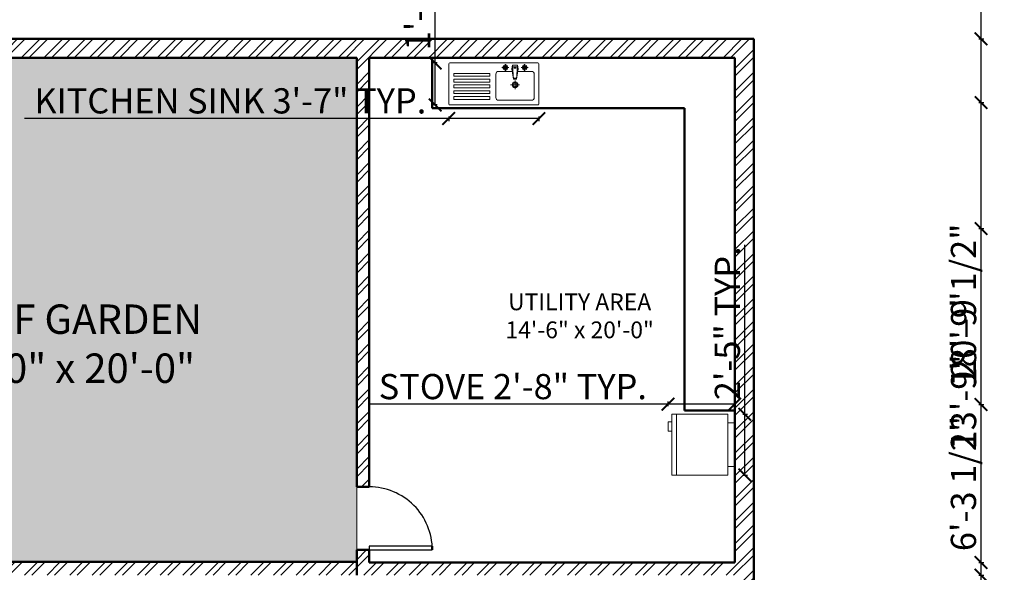
# Model space of a CAD drawing. Units: inches. Extents: x 261 to 2725, y 291 to 1454.
# Tile 34 of 35: x 2144 to 2613, y 801 to 1064. Entities that reach past the tile are written whole.
import ezdxf

# ---------------------------------------------------------------- set-up
doc = ezdxf.new("R2010")
doc.units = ezdxf.units.IN
for name, color, linetype, lineweight in [('A-ANNO-DIMS', 136, 'Continuous', 18), ('A-AREA-IDEN', 18, 'Continuous', 18), ('A-DOOR', 160, 'Continuous', 25), ('A-FLOR-FIXT', 145, 'Continuous', 18), ('A-PLNT', 3, 'Continuous', 18), ('A-PLNT-PATT', 3, 'Continuous', 13), ('A-WALL', 222, 'Continuous', 50), ('A-WALL-PATT', 243, 'Continuous', 13)]:
    doc.layers.add(name, color=color, linetype=linetype, lineweight=lineweight)
doc.styles.get("Standard").update_dxf_attribs({"font": 'arial.ttf'})
doc.dimstyles.new('ISO-25', dxfattribs={"dimtxt": 12, "dimasz": 6, "dimexe": 1.25, "dimexo": 0.625, "dimtad": 1, "dimdec": 0, "dimlunit": 3, "dimtxsty": 'Standard', "dimblk": 'ARCHTICK', "dimcen": 2.5, "dimadec": 0, "dimazin": 0, "dimtfac": 1, "dimtdec": 0, "dimtmove": 0, "dimatfit": 3, "dimfxl": 1, "dimfxlon": 1, "dimarcsym": 0})

# ---------------------------------------------------------------- blocks, each defined once
blk = doc.blocks.new('*U9')
for p, q in [((0, 0), (0, 6)), ((30, 0), (30, 6))]:
    blk.add_line(p, q)
blk.add_lwpolyline([(0, 0), (0, -30), (1.75, -30), (1.75, 0)], close=True)
blk.add_arc((0, 0), 30, 270, 0)
blk = doc.blocks.new('A$C7C492201')
for p, q in [((0, 10), (0, 427)), ((10, 437), (927, 437)), ((148, 425), (148, 352)), ((223, 415), (217, 376)), ((223, 415), (232, 268)), ((223, 415), (248, 415)), ((273, 415), (248, 415)), ((273, 415), (265, 268)), ((273, 415), (280, 376)), ((348, 425), (348, 352)), ((937, 10), (937, 427)), ((48, 319), (48, 79)), ((221, 349), (78, 349)), ((112, 389), (185, 389)), ((217, 376), (232, 268)), ((225, 395), (248, 395)), ((272, 395), (248, 395)), ((280, 376), (265, 268)), ((418, 349), (276, 349)), ((312, 389), (385, 389)), ((448, 319), (448, 79)), ((509, 328), (509, 298)), ((509, 328), (885, 328)), ((885, 328), (885, 298)), ((203, 208), (294, 208)), ((231, 279), (248, 279)), ((232, 268), (248, 268)), ((266, 279), (248, 279)), ((265, 268), (248, 268)), ((248, 253), (248, 163)), ((509, 298), (885, 298)), ((509, 268), (509, 238)), ((509, 268), (885, 268)), ((509, 238), (885, 238)), ((509, 208), (885, 208)), ((509, 208), (509, 178)), ((885, 268), (885, 238)), ((885, 208), (885, 178)), ((509, 178), (885, 178)), ((509, 148), (509, 118)), ((509, 148), (885, 148)), ((509, 118), (885, 118)), ((885, 148), (885, 118)), ((927, 0), (10, 0)), ((418, 49), (78, 49)), ((509, 88), (509, 58)), ((509, 88), (885, 88)), ((509, 58), (885, 58)), ((885, 88), (885, 58))]:
    blk.add_line(p, q)
for centre, radius in [((148, 389), 25), ((348, 389), 25), ((148, 389), 15), ((348, 389), 15), ((248, 208), 30), ((248, 208), 20)]:
    blk.add_circle(centre, radius)
for centre, radius, start, end in [((10, 427), 10, 90, 180), ((927, 427), 10, 0, 90), ((78, 319), 30, 90, 180), ((247, 388), 7.19, 80.5252, 279.4748), ((250, 388), 7.19, 260.5252, 99.4748), ((418, 319), 30, 0, 90), ((10, 10), 10, 180, 270), ((78, 79), 30, 180, 270), ((418, 79), 30, 270, 0), ((927, 10), 10, 270, 0)]:
    blk.add_arc(centre, radius, start, end)
blk = doc.blocks.new('A$C659B0DF6')
for p, q in [((585, 606.1), (0, 606.1)), ((0, 66.1), (0, 606.1)), ((423, 642.1), (423, 606.1)), ((513, 642.1), (423, 642.1)), ((513, 606.1), (513, 642.1)), ((585, 66.1), (585, 606.1)), ((585, 561.1), (0, 561.1)), ((0, 66.1), (585, 66.1)), ((82.3, 0), (82.3, 66.1)), ((502.7, 0), (502.7, 66.1)), ((82.3, 0), (502.7, 0))]:
    blk.add_line(p, q)
blk = doc.blocks.new('_ArchTick')
at = {"color": 0, "linetype": 'ByBlock', "const_width": 0.15}
blk.add_lwpolyline([(-0.5, -0.5), (0.5, 0.5)], dxfattribs=at)
blk = doc.blocks.new('*D51')
at = {"layer": 'A-ANNO-DIMS', "color": 0, "lineweight": -2, "ltscale": 0.07, "transparency": 16777216}
for p, q in [((2348.5, 1017.91), (2348.5, 1015.66)), ((2391.44, 1017.91), (2391.44, 1015.66)), ((2348.5, 1016.91), (2146.62, 1016.91)), ((2391.44, 1016.91), (2348.5, 1016.91))]:
    blk.add_line(p, q, dxfattribs=at)
at = {"layer": 'Defpoints', "color": 0, "ltscale": 0.07, "transparency": 16777216}
for p in [(2348.5, 1023.35), (2391.44, 1023.35), (2348.5, 1016.91)]:
    blk.add_point(p, dxfattribs=at)
at = {"layer": 'A-ANNO-DIMS', "color": 0, "lineweight": -2, "ltscale": 0.07, "transparency": 16777216, "xscale": 6, "yscale": 6, "zscale": 6, "rotation": 180}
blk.add_blockref('_ArchTick', (2348.5, 1016.91), dxfattribs=at)
at = {"layer": 'A-ANNO-DIMS', "color": 0, "lineweight": -2, "ltscale": 0.07, "transparency": 16777216, "xscale": 6, "yscale": 6, "zscale": 6}
blk.add_blockref('_ArchTick', (2391.44, 1016.91), dxfattribs=at)
at = {"layer": 'A-ANNO-DIMS', "color": 0, "ltscale": 0.07, "transparency": 16777216, "insert": (2244.56, 1023.75), "char_height": 12, "attachment_point": 5}
blk.add_mtext('KITCHEN SINK 3\'-7" TYP.', dxfattribs=at)
blk = doc.blocks.new('*D52')
at = {"layer": 'A-ANNO-DIMS', "color": 0, "lineweight": -2, "ltscale": 0.07, "transparency": 16777216}
for p, q in [((2342.06, 1043.35), (2342.06, 1122.62)), ((2343.06, 1043.35), (2340.81, 1043.35)), ((2342.06, 1023.35), (2342.06, 1043.35)), ((2343.06, 1023.35), (2340.81, 1023.35))]:
    blk.add_line(p, q, dxfattribs=at)
at = {"layer": 'Defpoints', "color": 0, "ltscale": 0.07, "transparency": 16777216}
for p in [(2342.06, 1043.35), (2348.5, 1043.35), (2348.5, 1023.35)]:
    blk.add_point(p, dxfattribs=at)
at = {"layer": 'A-ANNO-DIMS', "color": 0, "lineweight": -2, "ltscale": 0.07, "transparency": 16777216, "xscale": 6, "yscale": 6, "zscale": 6}
for p, rotation in [((2342.06, 1043.35), 90), ((2342.06, 1023.35), 270)]:
    blk.add_blockref('_ArchTick', p, dxfattribs=dict(at, rotation=rotation))
at = {"layer": 'A-ANNO-DIMS', "color": 0, "ltscale": 0.07, "transparency": 16777216, "insert": (2335.31, 1085.99), "char_height": 12, "attachment_point": 5, "rotation": 90}
blk.add_mtext('1\'-8" TYP.', dxfattribs=at)
blk = doc.blocks.new('*D53')
at = {"layer": 'A-ANNO-DIMS', "color": 0, "lineweight": -2, "ltscale": 0.07, "transparency": 16777216}
for p, q in [((2452.93, 879.86), (2452.93, 882.11)), ((2484.71, 879.86), (2484.71, 882.11)), ((2452.93, 880.86), (2311.11, 880.86)), ((2484.71, 880.86), (2452.93, 880.86))]:
    blk.add_line(p, q, dxfattribs=at)
at = {"layer": 'Defpoints', "color": 0, "ltscale": 0.07, "transparency": 16777216}
for p in [(2452.93, 880.86), (2452.93, 876.09), (2484.71, 876.09)]:
    blk.add_point(p, dxfattribs=at)
at = {"layer": 'A-ANNO-DIMS', "color": 0, "lineweight": -2, "ltscale": 0.07, "transparency": 16777216, "xscale": 6, "yscale": 6, "zscale": 6, "rotation": 180}
blk.add_blockref('_ArchTick', (2452.93, 880.86), dxfattribs=at)
at = {"layer": 'A-ANNO-DIMS', "color": 0, "lineweight": -2, "ltscale": 0.07, "transparency": 16777216, "xscale": 6, "yscale": 6, "zscale": 6}
blk.add_blockref('_ArchTick', (2484.71, 880.86), dxfattribs=at)
at = {"layer": 'A-ANNO-DIMS', "color": 0, "ltscale": 0.07, "transparency": 16777216, "insert": (2379.02, 887.69), "char_height": 12, "attachment_point": 5}
blk.add_mtext('STOVE 2\'-8" TYP.', dxfattribs=at)
blk = doc.blocks.new('*D54')
at = {"layer": 'A-ANNO-DIMS', "color": 0, "lineweight": -2, "ltscale": 0.07, "transparency": 16777216}
for p, q in [((2489.47, 876.09), (2489.47, 956.69)), ((2488.47, 876.09), (2490.72, 876.09)), ((2489.47, 847.13), (2489.47, 876.09)), ((2488.47, 847.13), (2490.72, 847.13))]:
    blk.add_line(p, q, dxfattribs=at)
at = {"layer": 'Defpoints', "color": 0, "ltscale": 0.07, "transparency": 16777216}
for p in [(2484.71, 876.09), (2489.47, 876.09), (2484.71, 847.13)]:
    blk.add_point(p, dxfattribs=at)
at = {"layer": 'A-ANNO-DIMS', "color": 0, "lineweight": -2, "ltscale": 0.07, "transparency": 16777216, "xscale": 6, "yscale": 6, "zscale": 6}
for p, rotation in [((2489.47, 876.09), 90), ((2489.47, 847.13), 270)]:
    blk.add_blockref('_ArchTick', p, dxfattribs=dict(at, rotation=rotation))
at = {"layer": 'A-ANNO-DIMS', "color": 0, "ltscale": 0.07, "transparency": 16777216, "insert": (2482.72, 919.39), "char_height": 12, "attachment_point": 5, "rotation": 90}
blk.add_mtext('2\'-5" TYP.', dxfattribs=at)
blk = doc.blocks.new('*D83')
at = {"layer": 'A-ANNO-DIMS', "color": 0, "lineweight": -2, "ltscale": 0.07, "transparency": 16777216}
for p, q in [((2600.96, 799.47), (2603.21, 799.47)), ((2601.96, 679.47), (2601.96, 799.47)), ((2600.96, 679.47), (2603.21, 679.47))]:
    blk.add_line(p, q, dxfattribs=at)
at = {"layer": 'Defpoints', "color": 0, "ltscale": 0.07, "transparency": 16777216}
for p in [(946.45, 799.47), (2601.96, 799.47), (946.45, 679.47)]:
    blk.add_point(p, dxfattribs=at)
at = {"layer": 'A-ANNO-DIMS', "color": 0, "lineweight": -2, "ltscale": 0.07, "transparency": 16777216, "xscale": 6, "yscale": 6, "zscale": 6}
for p, rotation in [((2601.96, 799.47), 90), ((2601.96, 679.47), 270)]:
    blk.add_blockref('_ArchTick', p, dxfattribs=dict(at, rotation=rotation))
at = {"layer": 'A-ANNO-DIMS', "color": 0, "ltscale": 0.07, "transparency": 16777216, "insert": (2595.21, 739.47), "char_height": 12, "attachment_point": 5, "rotation": 90}
blk.add_mtext('10\'-0"', dxfattribs=at)
blk = doc.blocks.new('*D84')
at = {"layer": 'A-ANNO-DIMS', "color": 0, "lineweight": -2, "ltscale": 0.07, "transparency": 16777216}
for p, q in [((2600.96, 1024.47), (2603.21, 1024.47)), ((2601.96, 799.47), (2601.96, 1024.47)), ((2600.96, 799.47), (2603.21, 799.47))]:
    blk.add_line(p, q, dxfattribs=at)
at = {"layer": 'Defpoints', "color": 0, "ltscale": 0.07, "transparency": 16777216}
for p in [(946.45, 1024.47), (2601.96, 1024.47), (946.45, 799.47)]:
    blk.add_point(p, dxfattribs=at)
at = {"layer": 'A-ANNO-DIMS', "color": 0, "lineweight": -2, "ltscale": 0.07, "transparency": 16777216, "xscale": 6, "yscale": 6, "zscale": 6}
for p, rotation in [((2601.96, 1024.47), 90), ((2601.96, 799.47), 270)]:
    blk.add_blockref('_ArchTick', p, dxfattribs=dict(at, rotation=rotation))
at = {"layer": 'A-ANNO-DIMS', "color": 0, "ltscale": 0.07, "transparency": 16777216, "insert": (2595.21, 911.97), "char_height": 12, "attachment_point": 5, "rotation": 90}
blk.add_mtext('18\'-9"', dxfattribs=at)
blk = doc.blocks.new('*D85')
at = {"layer": 'A-ANNO-DIMS', "color": 0, "lineweight": -2, "ltscale": 0.07, "transparency": 16777216}
for p, q in [((2600.96, 1222.47), (2603.21, 1222.47)), ((2601.96, 1024.47), (2601.96, 1222.47)), ((2600.96, 1024.47), (2603.21, 1024.47))]:
    blk.add_line(p, q, dxfattribs=at)
at = {"layer": 'Defpoints', "color": 0, "ltscale": 0.07, "transparency": 16777216}
for p in [(946.45, 1222.47), (2601.96, 1222.47), (946.45, 1024.47)]:
    blk.add_point(p, dxfattribs=at)
at = {"layer": 'A-ANNO-DIMS', "color": 0, "lineweight": -2, "ltscale": 0.07, "transparency": 16777216, "xscale": 6, "yscale": 6, "zscale": 6}
for p, rotation in [((2601.96, 1222.47), 90), ((2601.96, 1024.47), 270)]:
    blk.add_blockref('_ArchTick', p, dxfattribs=dict(at, rotation=rotation))
at = {"layer": 'A-ANNO-DIMS', "color": 0, "ltscale": 0.07, "transparency": 16777216, "insert": (2595.21, 1123.47), "char_height": 12, "attachment_point": 5, "rotation": 90}
blk.add_mtext('16\'-6"', dxfattribs=at)
blk = doc.blocks.new('*D113')
at = {"layer": 'A-ANNO-DIMS', "color": 0, "lineweight": -2, "ltscale": 0.07, "transparency": 16777216}
for p, q in [((2600.96, 799.47), (2603.21, 799.47)), ((2601.96, 679.47), (2601.96, 799.47)), ((2600.96, 679.47), (2603.21, 679.47))]:
    blk.add_line(p, q, dxfattribs=at)
at = {"layer": 'Defpoints', "color": 0, "ltscale": 0.07, "transparency": 16777216}
for p in [(1720.08, 799.47), (2601.96, 799.47), (1720.08, 679.47)]:
    blk.add_point(p, dxfattribs=at)
at = {"layer": 'A-ANNO-DIMS', "color": 0, "lineweight": -2, "ltscale": 0.07, "transparency": 16777216, "xscale": 6, "yscale": 6, "zscale": 6}
for p, rotation in [((2601.96, 799.47), 90), ((2601.96, 679.47), 270)]:
    blk.add_blockref('_ArchTick', p, dxfattribs=dict(at, rotation=rotation))
at = {"layer": 'A-ANNO-DIMS', "color": 0, "ltscale": 0.07, "transparency": 16777216, "insert": (2595.21, 739.47), "char_height": 12, "attachment_point": 5, "rotation": 90}
blk.add_mtext('10\'-0"', dxfattribs=at)
blk = doc.blocks.new('*D114')
at = {"layer": 'A-ANNO-DIMS', "color": 0, "lineweight": -2, "ltscale": 0.07, "transparency": 16777216}
for p, q in [((2600.96, 964.47), (2603.21, 964.47)), ((2601.96, 799.47), (2601.96, 964.47)), ((2600.96, 799.47), (2603.21, 799.47))]:
    blk.add_line(p, q, dxfattribs=at)
at = {"layer": 'Defpoints', "color": 0, "ltscale": 0.07, "transparency": 16777216}
for p in [(1720.08, 964.47), (2601.96, 964.47), (1720.08, 799.47)]:
    blk.add_point(p, dxfattribs=at)
at = {"layer": 'A-ANNO-DIMS', "color": 0, "lineweight": -2, "ltscale": 0.07, "transparency": 16777216, "xscale": 6, "yscale": 6, "zscale": 6}
for p, rotation in [((2601.96, 964.47), 90), ((2601.96, 799.47), 270)]:
    blk.add_blockref('_ArchTick', p, dxfattribs=dict(at, rotation=rotation))
at = {"layer": 'A-ANNO-DIMS', "color": 0, "ltscale": 0.07, "transparency": 16777216, "insert": (2595.2, 881.97), "char_height": 12, "attachment_point": 5, "rotation": 90}
blk.add_mtext('13\'-9"', dxfattribs=at)
blk = doc.blocks.new('*D115')
at = {"layer": 'A-ANNO-DIMS', "color": 0, "lineweight": -2, "ltscale": 0.07, "transparency": 16777216}
for p, q in [((2600.96, 1222.47), (2603.21, 1222.47)), ((2601.96, 964.47), (2601.96, 1222.47)), ((2600.96, 964.47), (2603.21, 964.47))]:
    blk.add_line(p, q, dxfattribs=at)
at = {"layer": 'Defpoints', "color": 0, "ltscale": 0.07, "transparency": 16777216}
for p in [(1720.08, 1222.47), (2601.96, 1222.47), (1720.08, 964.47)]:
    blk.add_point(p, dxfattribs=at)
at = {"layer": 'A-ANNO-DIMS', "color": 0, "lineweight": -2, "ltscale": 0.07, "transparency": 16777216, "xscale": 6, "yscale": 6, "zscale": 6}
for p, rotation in [((2601.96, 1222.47), 90), ((2601.96, 964.47), 270)]:
    blk.add_blockref('_ArchTick', p, dxfattribs=dict(at, rotation=rotation))
at = {"layer": 'A-ANNO-DIMS', "color": 0, "ltscale": 0.07, "transparency": 16777216, "insert": (2595.21, 1093.47), "char_height": 12, "attachment_point": 5, "rotation": 90}
blk.add_mtext('21\'-6"', dxfattribs=at)
blk = doc.blocks.new('*D120')
at = {"layer": 'A-ANNO-DIMS', "color": 0, "lineweight": -2, "ltscale": 0.07, "transparency": 16777216}
for p, q in [((2600.96, 880.73), (2603.21, 880.73)), ((2601.96, 805.47), (2601.96, 880.73)), ((2600.96, 805.47), (2603.21, 805.47))]:
    blk.add_line(p, q, dxfattribs=at)
at = {"layer": 'Defpoints', "color": 0, "ltscale": 0.07, "transparency": 16777216}
for p in [(1559.08, 880.73), (2601.96, 880.73), (1558.08, 805.47)]:
    blk.add_point(p, dxfattribs=at)
at = {"layer": 'A-ANNO-DIMS', "color": 0, "lineweight": -2, "ltscale": 0.07, "transparency": 16777216, "xscale": 6, "yscale": 6, "zscale": 6}
for p, rotation in [((2601.96, 880.73), 90), ((2601.96, 805.47), 270)]:
    blk.add_blockref('_ArchTick', p, dxfattribs=dict(at, rotation=rotation))
at = {"layer": 'A-ANNO-DIMS', "color": 0, "ltscale": 0.07, "transparency": 16777216, "insert": (2595.12, 843.1), "char_height": 12, "attachment_point": 5, "rotation": 90}
blk.add_mtext('6\'-3 1/2"', dxfattribs=at)
blk = doc.blocks.new('*D122')
at = {"layer": 'A-ANNO-DIMS', "color": 0, "lineweight": -2, "ltscale": 0.07, "transparency": 16777216}
for p, q in [((2007.71, 1437.76), (2007.71, 1440.01)), ((2493.71, 1437.76), (2493.71, 1440.01)), ((2007.71, 1438.76), (2493.71, 1438.76))]:
    blk.add_line(p, q, dxfattribs=at)
at = {"layer": 'Defpoints', "color": 0, "ltscale": 0.07, "transparency": 16777216}
for p in [(2493.71, 1438.76), (2007.71, 1054.85), (2493.71, 1054.85)]:
    blk.add_point(p, dxfattribs=at)
at = {"layer": 'A-ANNO-DIMS', "color": 0, "lineweight": -2, "ltscale": 0.07, "transparency": 16777216, "xscale": 6, "yscale": 6, "zscale": 6, "rotation": 180}
blk.add_blockref('_ArchTick', (2007.71, 1438.76), dxfattribs=at)
at = {"layer": 'A-ANNO-DIMS', "color": 0, "lineweight": -2, "ltscale": 0.07, "transparency": 16777216, "xscale": 6, "yscale": 6, "zscale": 6}
blk.add_blockref('_ArchTick', (2493.71, 1438.76), dxfattribs=at)
at = {"layer": 'A-ANNO-DIMS', "color": 0, "ltscale": 0.07, "transparency": 16777216, "insert": (2250.71, 1445.51), "char_height": 12, "attachment_point": 5}
blk.add_mtext('40\'-6"', dxfattribs=at)
blk = doc.blocks.new('*D127')
at = {"layer": 'A-ANNO-DIMS', "color": 0, "lineweight": -2, "ltscale": 0.07, "transparency": 16777216}
for p, q in [((2600.96, 805.47), (2603.21, 805.47)), ((2601.96, 673.47), (2601.96, 805.47)), ((2600.96, 673.47), (2603.21, 673.47))]:
    blk.add_line(p, q, dxfattribs=at)
at = {"layer": 'Defpoints', "color": 0, "ltscale": 0.07, "transparency": 16777216}
for p in [(2484.71, 805.47), (2601.96, 805.47), (2484.71, 673.47)]:
    blk.add_point(p, dxfattribs=at)
at = {"layer": 'A-ANNO-DIMS', "color": 0, "lineweight": -2, "ltscale": 0.07, "transparency": 16777216, "xscale": 6, "yscale": 6, "zscale": 6}
for p, rotation in [((2601.96, 805.47), 90), ((2601.96, 673.47), 270)]:
    blk.add_blockref('_ArchTick', p, dxfattribs=dict(at, rotation=rotation))
at = {"layer": 'A-ANNO-DIMS', "color": 0, "ltscale": 0.07, "transparency": 16777216, "insert": (2595.21, 739.47), "char_height": 12, "attachment_point": 5, "rotation": 90}
blk.add_mtext('11\'-0"', dxfattribs=at)
blk = doc.blocks.new('*D128')
at = {"layer": 'A-ANNO-DIMS', "color": 0, "lineweight": -2, "ltscale": 0.07, "transparency": 16777216}
for p, q in [((2600.96, 1054.85), (2603.21, 1054.85)), ((2601.96, 805.47), (2601.96, 1054.85)), ((2600.96, 805.47), (2603.21, 805.47))]:
    blk.add_line(p, q, dxfattribs=at)
at = {"layer": 'Defpoints', "color": 0, "ltscale": 0.07, "transparency": 16777216}
for p in [(2493.71, 1054.85), (2601.96, 1054.85), (2484.71, 805.47)]:
    blk.add_point(p, dxfattribs=at)
at = {"layer": 'A-ANNO-DIMS', "color": 0, "lineweight": -2, "ltscale": 0.07, "transparency": 16777216, "xscale": 6, "yscale": 6, "zscale": 6}
for p, rotation in [((2601.96, 1054.85), 90), ((2601.96, 805.47), 270)]:
    blk.add_blockref('_ArchTick', p, dxfattribs=dict(at, rotation=rotation))
at = {"layer": 'A-ANNO-DIMS', "color": 0, "ltscale": 0.07, "transparency": 16777216, "insert": (2595.13, 930.16), "char_height": 12, "attachment_point": 5, "rotation": 90}
blk.add_mtext('20\'-9 1/2"', dxfattribs=at)
blk = doc.blocks.new('*D135')
at = {"layer": 'A-ANNO-DIMS', "color": 0, "lineweight": -2, "ltscale": 0.07, "transparency": 16777216}
for p, q in [((2004.19, 1437.76), (2004.19, 1440.01)), ((2221.19, 1437.76), (2221.19, 1440.01)), ((2004.19, 1438.76), (2221.19, 1438.76))]:
    blk.add_line(p, q, dxfattribs=at)
at = {"layer": 'Defpoints', "color": 0, "ltscale": 0.07, "transparency": 16777216}
for p in [(2221.19, 1438.76), (2004.19, 642.39), (2221.19, 642.39)]:
    blk.add_point(p, dxfattribs=at)
at = {"layer": 'A-ANNO-DIMS', "color": 0, "lineweight": -2, "ltscale": 0.07, "transparency": 16777216, "xscale": 6, "yscale": 6, "zscale": 6, "rotation": 180}
blk.add_blockref('_ArchTick', (2004.19, 1438.76), dxfattribs=at)
at = {"layer": 'A-ANNO-DIMS', "color": 0, "lineweight": -2, "ltscale": 0.07, "transparency": 16777216, "xscale": 6, "yscale": 6, "zscale": 6}
blk.add_blockref('_ArchTick', (2221.19, 1438.76), dxfattribs=at)
at = {"layer": 'A-ANNO-DIMS', "color": 0, "ltscale": 0.07, "transparency": 16777216, "insert": (2112.69, 1445.51), "char_height": 12, "attachment_point": 5}
blk.add_mtext('18\'-1"', dxfattribs=at)

msp = doc.modelspace()

# ---------------------------------------------------------------- hatches: boundary and pattern name
at = {"layer": 'A-PLNT-PATT'}
h = msp.add_hatch(dxfattribs=at)
h.set_pattern_fill('GRASS', color=256, scale=0.7)
h.paths.add_polyline_path([(658.45, 427.47), (433.45, 427.47), (433.45, 415.47), (658.45, 415.47)])
h.paths.add_polyline_path([(670.45, 421.47), (664.45, 421.47), (664.45, 415.47), (670.45, 415.47)])
h.paths.add_polyline_path([(784.45, 421.47), (778.45, 421.47), (778.45, 415.47), (784.45, 415.47)])
h.paths.add_polyline_path([(991.45, 427.47), (790.45, 427.47), (790.45, 415.47), (991.45, 415.47)])
h.paths.add_polyline_path([(1439.08, 1220.47), (1252.08, 1220.47), (1252.08, 1198.47), (1417.08, 1198.47), (1417.08, 1117.47), (1439.08, 1117.47)])
h.paths.add_polyline_path([(2304.71, 1045.85), (2016.71, 1045.85), (2016.71, 805.87), (2304.71, 805.87)])
h.paths.add_polyline_path([(1267.21, 1201.68), (1431.59, 1201.68), (1431.59, 1218.76), (1267.21, 1218.76)], flags=24)
h.paths.add_polyline_path([(2089.2, 883.04), (2242.64, 883.04), (2242.64, 936.27), (2089.2, 936.27)], flags=24)
at = {"layer": 'A-WALL-PATT'}
h = msp.add_hatch(dxfattribs=at)
h.set_pattern_fill('ANSI32', color=256, scale=0.8)
h.paths.add_polyline_path([(478.45, 685.47), (580.45, 685.47), (580.45, 691.47), (577.45, 691.47), (577.45, 694.47), (571.45, 694.47), (571.45, 691.47), (478.45, 691.47), (478.45, 721.47), (469.45, 721.47), (469.45, 508.47), (538.45, 508.47), (538.45, 517.47), (478.45, 517.47)])
h.paths.add_polyline_path([(694.45, 517.47), (676.45, 517.47), (676.45, 646.47), (670.45, 646.47), (670.45, 517.47), (610.45, 517.47), (610.45, 508.47), (694.45, 508.47)])
h.paths.add_polyline_path([(676.45, 784.47), (478.45, 784.47), (478.45, 844.47), (469.45, 844.47), (469.45, 745.47), (478.45, 745.47), (478.45, 775.47), (571.45, 775.47), (571.45, 724.47), (577.45, 724.47), (577.45, 775.47), (670.45, 775.47), (670.45, 691.47), (610.45, 691.47), (610.45, 685.47), (670.45, 685.47), (670.45, 682.47), (676.45, 682.47)])
h.paths.add_polyline_path([(955.45, 880.47), (946.45, 880.47), (946.45, 808.47), (778.45, 808.47), (778.45, 799.47), (946.45, 799.47), (946.45, 517.47), (898.45, 517.47), (898.45, 508.47), (955.45, 508.47)])
h.paths.add_polyline_path([(778.45, 598.47), (772.45, 598.47), (772.45, 517.47), (754.45, 517.47), (754.45, 508.47), (826.45, 508.47), (826.45, 517.47), (778.45, 517.47)])
h.paths.add_polyline_path([(955.45, 1090.47), (946.45, 1090.47), (946.45, 1030.47), (817.45, 1030.47), (817.45, 1024.47), (946.45, 1024.47), (946.45, 952.47), (955.45, 952.47)])
h.paths.add_polyline_path([(955.45, 1231.47), (730.45, 1231.47), (730.45, 1222.47), (772.45, 1222.47), (772.45, 1096.47), (766.45, 1096.47), (766.45, 1090.47), (772.45, 1090.47), (772.45, 1006.47), (712.45, 1006.47), (712.45, 1000.47), (778.45, 1000.47), (778.45, 1024.47), (781.45, 1024.47), (781.45, 1030.47), (778.45, 1030.47), (778.45, 1222.47), (946.45, 1222.47), (946.45, 1162.47), (955.45, 1162.47)])
h.paths.add_polyline_path([(694.45, 1231.47), (619.45, 1231.47), (619.45, 1222.47), (646.45, 1222.47), (646.45, 1039.47), (652.45, 1039.47), (652.45, 1090.47), (736.45, 1090.47), (736.45, 1096.47), (652.45, 1096.47), (652.45, 1222.47), (694.45, 1222.47)])
h.paths.add_polyline_path([(571.45, 1231.47), (469.45, 1231.47), (469.45, 1099.47), (478.45, 1099.47), (478.45, 1144.47), (544.45, 1144.47), (544.45, 1153.47), (538.45, 1153.47), (538.45, 1150.47), (478.45, 1150.47), (478.45, 1222.47), (538.45, 1222.47), (538.45, 1183.47), (544.45, 1183.47), (544.45, 1222.47), (571.45, 1222.47)])
h.paths.add_polyline_path([(538.45, 1006.47), (478.45, 1006.47), (478.45, 1051.47), (469.45, 1051.47), (469.45, 940.47), (478.45, 940.47), (478.45, 1000.47), (538.45, 1000.47)])
h.paths.add_polyline_path([(652.45, 1006.47), (652.45, 1009.47), (646.45, 1009.47), (646.45, 1006.47), (586.45, 1006.47), (586.45, 1000.47), (652.45, 1000.47)])
h.paths.add_polyline_path([(1288.08, 973.47), (1243.08, 973.47), (1243.08, 920.97), (1252.08, 920.97), (1252.08, 964.47), (1288.08, 964.47)], flags=17)
h.paths.add_polyline_path([(1402.08, 805.47), (1252.08, 805.47), (1252.08, 848.97), (1243.08, 848.97), (1243.08, 757.47), (1252.08, 757.47), (1252.08, 799.47), (1294.08, 799.47), (1372.08, 799.47), (1372.08, 779.47), (1372.08, 715.47), (1378.08, 715.47), (1378.08, 799.47), (1402.08, 799.47)])
h.paths.add_polyline_path([(1252.08, 721.47), (1243.08, 721.47), (1243.08, 439.47), (1729.08, 439.47), (1729.08, 709.47), (1720.08, 709.47), (1720.08, 679.47), (1582.08, 679.47), (1582.08, 670.47), (1588.08, 670.47), (1588.08, 673.47), (1720.08, 673.47), (1720.08, 559.47), (1690.08, 559.47), (1690.08, 550.47), (1720.08, 550.47), (1720.08, 448.47), (1252.08, 448.47), (1252.08, 496.47), (1312.08, 496.47), (1312.08, 505.47), (1252.08, 505.47), (1252.08, 673.47), (1405.08, 673.47), (1405.08, 679.47), (1378.08, 679.47), (1378.08, 685.47), (1372.08, 685.47), (1372.08, 679.47), (1252.08, 679.47)])
h.paths.add_polyline_path([(1450.08, 550.47), (1480.08, 550.47), (1480.08, 559.47), (1450.08, 559.47), (1450.08, 679.47), (1441.08, 679.47), (1441.08, 673.47), (1444.08, 673.47), (1444.08, 505.47), (1384.08, 505.47), (1384.08, 496.47), (1450.08, 496.47)], flags=17)
h.paths.add_polyline_path([(1618.08, 559.47), (1588.08, 559.47), (1588.08, 634.47), (1582.08, 634.47), (1582.08, 559.47), (1552.08, 559.47), (1552.08, 550.47), (1618.08, 550.47)], flags=17)
h.paths.add_polyline_path([(1564.08, 964.47), (1630.08, 964.47), (1630.08, 973.47), (1477.08, 973.47), (1477.08, 964.47), (1558.08, 964.47), (1558.08, 926.22), (1558.08, 887.97), (1486.08, 887.97), (1486.08, 881.97), (1558.08, 881.97), (1558.08, 805.47), (1450.08, 805.47), (1450.08, 845.97), (1444.08, 845.97), (1444.08, 805.47), (1438.08, 805.47), (1438.08, 799.47), (1564.08, 799.47)], flags=17)
h.paths.add_polyline_path([(1453.08, 973.47), (1408.08, 973.47), (1408.08, 964.47), (1444.08, 964.47), (1444.08, 881.97), (1450.08, 881.97), (1456.08, 881.97), (1456.08, 887.97), (1450.08, 887.97), (1450.08, 964.47), (1453.08, 964.47)], flags=17)
h.paths.add_polyline_path([(1729.08, 1231.47), (1243.08, 1231.47), (1243.08, 1167.47), (1252.08, 1167.47), (1252.08, 1222.47), (1441.08, 1222.47), (1441.08, 1045.47), (1648.08, 1045.47), (1648.08, 1051.47), (1450.08, 1051.47), (1450.08, 1074.47), (1450.08, 1222.47), (1472.08, 1222.47), (1720.08, 1222.47), (1720.08, 1051.47), (1708.08, 1051.47), (1708.08, 1045.47), (1720.08, 1045.47), (1720.08, 973.47), (1702.08, 973.47), (1702.08, 964.47), (1720.08, 964.47), (1720.08, 769.47), (1729.08, 769.47)])
h.paths.add_polyline_path([(2493.71, 1054.85), (2007.71, 1054.85), (2007.71, 439.47), (2214.67, 439.47), (2214.67, 496.47), (2493.71, 496.47)])
h.paths.add_polyline_path([(2016.71, 1045.85), (2304.71, 1045.85), (2304.71, 841.47), (2310.71, 841.47), (2310.71, 1045.85), (2484.71, 1045.85), (2484.71, 805.47), (2310.71, 805.47), (2310.71, 811.47), (2304.71, 811.47), (2304.71, 799.47), (2484.71, 799.47), (2484.71, 679.47), (2304.71, 679.47), (2304.71, 673.47), (2484.71, 673.47), (2484.71, 505.47), (2208.67, 505.47), (2208.67, 448.47), (2016.71, 448.47), (2016.71, 799.47), (2304.71, 799.47), (2304.71, 805.47), (2016.71, 805.47)], flags=16)

# ---------------------------------------------------------------- linework, layer by layer
at = {"layer": 'A-PLNT'}
msp.add_lwpolyline([(2016.71, 1045.85), (2304.71, 1045.85), (2304.71, 805.87), (2016.71, 805.87)], close=True, dxfattribs=at)
at = {"layer": 'A-WALL'}
for p, q in [((2007.71, 1054.85), (2493.71, 1054.85)), ((2493.71, 1054.85), (2493.71, 496.47)), ((2016.71, 1045.85), (2304.71, 1045.85)), ((2304.71, 1045.85), (2304.71, 841.47)), ((2310.71, 1045.85), (2310.71, 841.47)), ((2310.71, 1045.85), (2484.71, 1045.85)), ((2340.71, 1045.85), (2340.71, 1021.85)), ((2484.71, 1045.85), (2484.71, 805.47)), ((2340.71, 1021.85), (2460.71, 1021.85)), ((2460.71, 1021.85), (2460.71, 877.85)), ((2460.71, 877.85), (2484.71, 877.85)), ((2310.71, 841.47), (2304.71, 841.47)), ((2310.71, 811.47), (2304.71, 811.47)), ((2304.71, 811.47), (2304.71, 799.47)), ((2310.71, 811.47), (2310.71, 805.47)), ((2340.71, 813.22), (2340.71, 811.47)), ((2016.71, 805.87), (2304.71, 805.87)), ((2310.71, 805.47), (2484.71, 805.47))]:
    msp.add_line(p, q, dxfattribs=at)

# ---------------------------------------------------------------- block references
at = {"layer": 'A-DOOR', "rotation": 89.99999999999999}
msp.add_blockref('*U9', (2310.71, 811.47), dxfattribs=at)
at = {"layer": 'A-FLOR-FIXT', "xscale": -0.0458075162661089, "yscale": 0.0458075162661089, "zscale": 0.0458075162661089}
msp.add_blockref('A$C7C492201', (2391.44, 1023.35), dxfattribs=at)
at = {"layer": 'A-FLOR-FIXT', "xscale": 0.049496254826062, "yscale": 0.049496254826062, "zscale": 0.049496254826062, "rotation": 89.99999999999999}
msp.add_blockref('A$C659B0DF6', (2484.71, 847.13), dxfattribs=at)

# ---------------------------------------------------------------- texts
at = {"layer": 'A-AREA-IDEN', "attachment_point": 1}
for s, width, insert, char_height in [('\\pxqc;{\\fTimes New Roman|b0|i0|c0|p18;UTILITY AREA\\P14\'-6" x 20\'-0"}', 88.8228, (2366.44, 933.6), 8), ('\\pxqc;{\\fTimes New Roman|b0|i0|c0|p18;ROOF GARDEN\\P24\'-0" x 20\'-0"}', 148.4764, (2091.71, 928.35), 14)]:
    msp.add_mtext_dynamic_manual_height_columns(s, width=width, gutter_width=12.5, heights=[0], dxfattribs=dict(at, insert=insert, char_height=char_height))

# ---------------------------------------------------------------- dimensions: what is measured, and where the dimension line sits
at = {"layer": 'A-ANNO-DIMS', "ltscale": 0.07}
for base, p1, p2, picture, middle in [((2221.19, 1438.76), (2004.19, 642.39), (2221.19, 642.39), '*D135', (2112.69, 1445.51)), ((2493.71, 1438.76), (2007.71, 1054.85), (2493.71, 1054.85), '*D122', (2250.71, 1445.51))]:
    dim = msp.add_linear_dim(base=base, p1=p1, p2=p2, dimstyle='ISO-25', override={"dimdec": 1, "dimlfac": 1, "dimrnd": 0, "dimzin": 1, "dimdsep": 46, "dimlunit": 4, "dimfrac": 2}, dxfattribs=at)
    dim.commit()
    dim.dimension.update_dxf_attribs({"geometry": picture, "text_midpoint": middle})
for base, p1, p2, picture, middle in [((2601.96, 1222.47), (946.45, 1024.47), (946.45, 1222.47), '*D85', (2595.21, 1123.47)), ((2601.96, 1222.47), (1720.08, 964.47), (1720.08, 1222.47), '*D115', (2595.21, 1093.47)), ((2601.96, 1054.85), (2484.71, 805.47), (2493.71, 1054.85), '*D128', (2595.13, 930.16)), ((2601.96, 1024.47), (946.45, 799.47), (946.45, 1024.47), '*D84', (2595.21, 911.97)), ((2601.96, 964.47), (1720.08, 799.47), (1720.08, 964.47), '*D114', (2595.2, 881.97)), ((2601.96, 880.73), (1558.08, 805.47), (1559.08, 880.73), '*D120', (2595.12, 843.1)), ((2601.96, 805.47), (2484.71, 673.47), (2484.71, 805.47), '*D127', (2595.21, 739.47)), ((2601.96, 799.47), (946.45, 679.47), (946.45, 799.47), '*D83', (2595.21, 739.47)), ((2601.96, 799.47), (1720.08, 679.47), (1720.08, 799.47), '*D113', (2595.21, 739.47))]:
    dim = msp.add_linear_dim(base=base, p1=p1, p2=p2, angle=90, dimstyle='ISO-25', override={"dimdec": 1, "dimlfac": 1, "dimrnd": 0, "dimzin": 1, "dimdsep": 46, "dimlunit": 4, "dimfrac": 2}, dxfattribs=at)
    dim.commit()
    dim.dimension.update_dxf_attribs({"geometry": picture, "text_midpoint": middle})
for base, p1, p2, angle, text, picture, middle in [((2342.06, 1043.35), (2348.5, 1023.35), (2348.5, 1043.35), 90, '<> TYP.', '*D52', (2335.31, 1085.99)), ((2348.5, 1016.91), (2391.44, 1023.35), (2348.5, 1023.35), 180, 'KITCHEN SINK <> TYP.', '*D51', (2244.56, 1023.75)), ((2489.47, 876.09), (2484.71, 847.13), (2484.71, 876.09), 90, '<> TYP.', '*D54', (2482.72, 919.39)), ((2452.93, 880.86), (2484.71, 876.09), (2452.93, 876.09), 180, 'STOVE <> TYP.', '*D53', (2379.02, 887.69))]:
    dim = msp.add_linear_dim(base=base, p1=p1, p2=p2, angle=angle, text=text, dimstyle='ISO-25', override={"dimdec": 1, "dimrnd": 0, "dimzin": 1, "dimlunit": 4, "dimfrac": 2}, dxfattribs=at)
    dim.commit()
    dim.dimension.update_dxf_attribs({"geometry": picture, "text_midpoint": middle})

doc.saveas('drawing.dxf')
